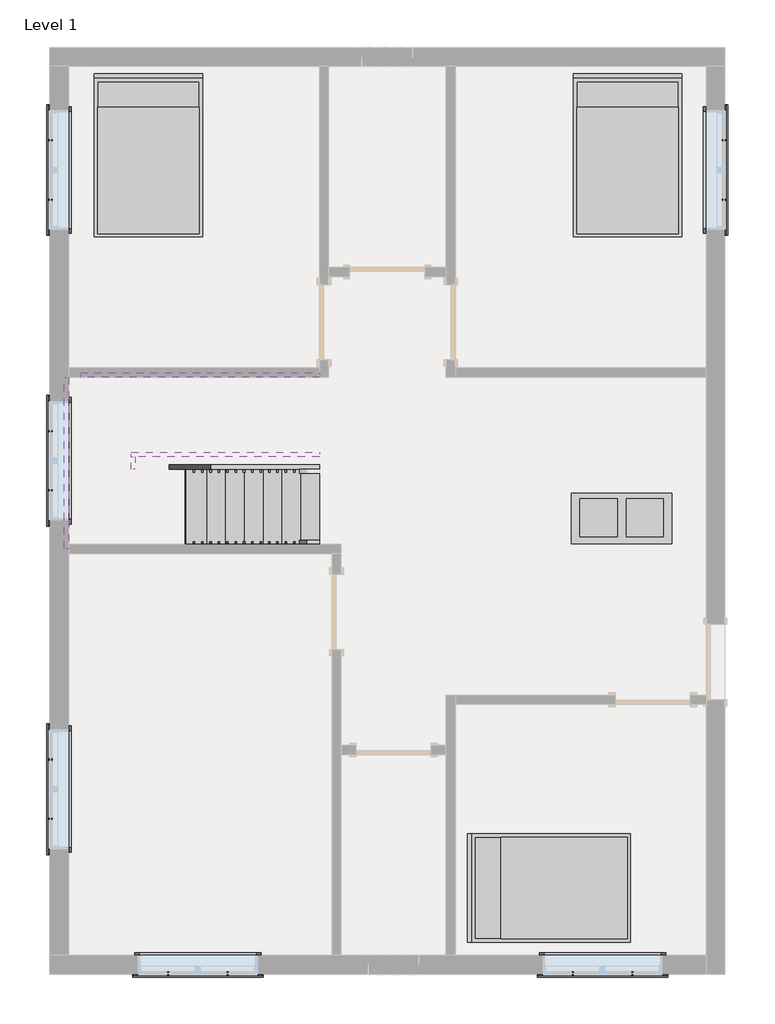
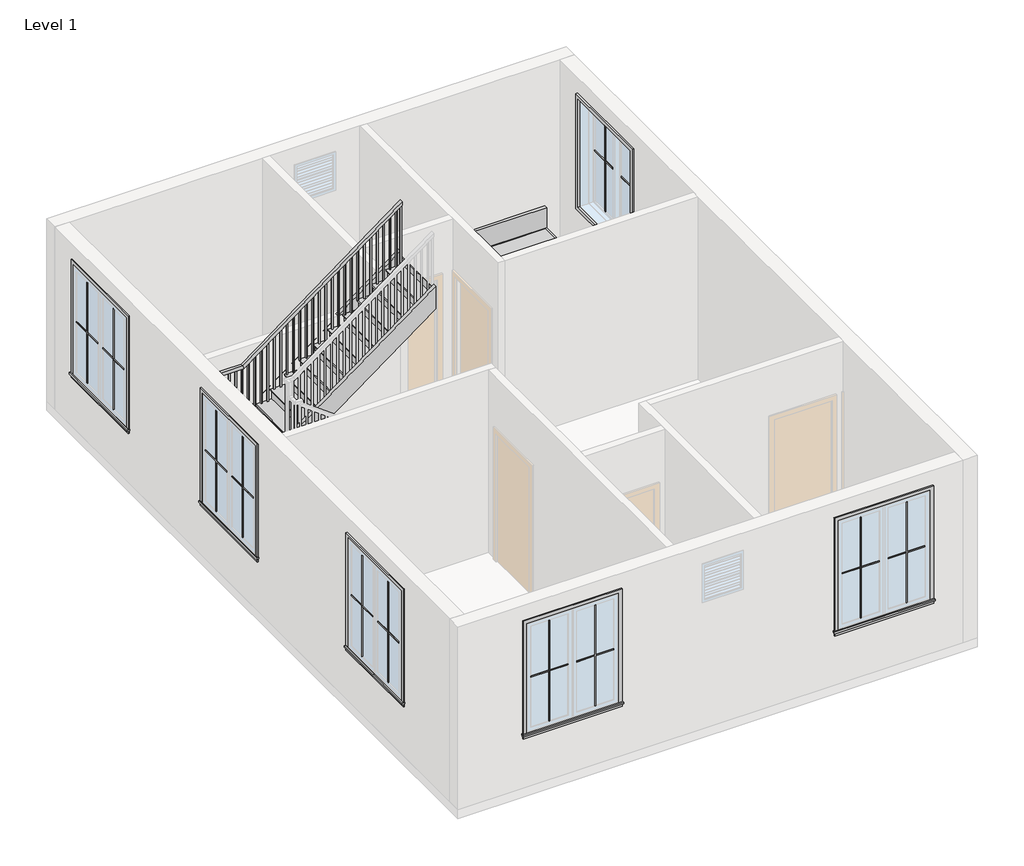
# One storey, part 2 of 2: 25 proxies, 6 members, 3 furniture elements, 1 railing, 1 stair flight.
"""IFC4 building model written with IfcOpenShell, lengths in millimetres."""

from ifc_helpers import new_model, si_unit, frame, origin, place, context, project, spatial, polyline, outline, extrude, faceted_brep, transform, mapped, element, save
from components import muntin_pattern_2x2_muntin_pattern_2x2_bff912c5, muntin_pattern_2x2_muntin_pattern_2x2_c2194282, trim_window_exterior_flat_with_sill_e04b3088, trim_window_interior_flat_picture_frame_2a7685fe, coffee_table_with_brass_mullions_11320_coffee_table_with_5962bef7, bed_17739_bed_17739_15c61121, stair_flight_66f938e6

model = new_model("IFC4")

# Units and contexts
model_context = context("Model", 3, world=origin())
ifc_project = project(units=[si_unit("LENGTHUNIT", "METRE", prefix="MILLI")], contexts=[model_context])

# Site, building, storey
site = spatial("IfcSite", under=ifc_project)
building = spatial("IfcBuilding", under=site)
storey = spatial("IfcBuildingStorey", under=building, Name="Level 1", Elevation=0.0)

# Proxies
placement = place(None, origin())
muntin_pattern_2x2_muntin_pattern_2x2_shape = muntin_pattern_2x2_muntin_pattern_2x2_bff912c5(model_context)
element("IfcBuildingElementProxy", 1, Name="Muntin Pattern_2x2 : Muntin Pattern_2x2", ObjectType="Muntin Pattern_2x2 : Muntin Pattern_2x2", at=placement, inside=storey, context=model_context, shape_type="MappedRepresentation", body=[
    mapped(muntin_pattern_2x2_muntin_pattern_2x2_shape, transform((-3196.8535855, -5792.3946383, 984.25), x_axis=(-1.0, 0.0, 0.0), y_axis=(0.0, -1.0, 0.0), z_axis=(0.0, 0.0, 1.0))),
])
element("IfcBuildingElementProxy", 2, Name="Muntin Pattern_2x2 : Muntin Pattern_2x2", ObjectType="Muntin Pattern_2x2 : Muntin Pattern_2x2", at=placement, inside=storey, context=model_context, shape_type="MappedRepresentation", body=[
    mapped(muntin_pattern_2x2_muntin_pattern_2x2_shape, transform((-5347.9160855, -3914.3821383, 984.25), x_axis=(0.0, 1.0, 0.0), y_axis=(-1.0, 0.0, 0.0), z_axis=(0.0, 0.0, 1.0))),
])
element("IfcBuildingElementProxy", 3, Name="Muntin Pattern_2x2 : Muntin Pattern_2x2", ObjectType="Muntin Pattern_2x2 : Muntin Pattern_2x2", at=placement, inside=storey, context=model_context, shape_type="MappedRepresentation", body=[
    mapped(muntin_pattern_2x2_muntin_pattern_2x2_shape, transform((1721.2214145, -5792.3946383, 984.25), x_axis=(-1.0, 0.0, 0.0), y_axis=(0.0, -1.0, 0.0), z_axis=(0.0, 0.0, 1.0))),
])
element("IfcBuildingElementProxy", 4, Name="Muntin Pattern_2x2 : Muntin Pattern_2x2", ObjectType="Muntin Pattern_2x2 : Muntin Pattern_2x2", at=placement, inside=storey, context=model_context, shape_type="MappedRepresentation", body=[
    mapped(muntin_pattern_2x2_muntin_pattern_2x2_shape, transform((2837.2339145, 4324.7428617, 984.25), x_axis=(0.0, -1.0, 0.0), y_axis=(1.0, 0.0, 0.0), z_axis=(0.0, 0.0, 1.0))),
])
element("IfcBuildingElementProxy", 5, Name="Muntin Pattern_2x2 : Muntin Pattern_2x2", ObjectType="Muntin Pattern_2x2 : Muntin Pattern_2x2", at=placement, inside=storey, context=model_context, shape_type="MappedRepresentation", body=[
    mapped(muntin_pattern_2x2_muntin_pattern_2x2_shape, transform((-5347.9160855, 3604.0178617, 984.25), x_axis=(0.0, 1.0, 0.0), y_axis=(-1.0, 0.0, 0.0), z_axis=(0.0, 0.0, 1.0))),
])
element("IfcBuildingElementProxy", 6, Name="Muntin Pattern_2x2 : Muntin Pattern_2x2", ObjectType="Muntin Pattern_2x2 : Muntin Pattern_2x2", at=placement, inside=storey, context=model_context, shape_type="MappedRepresentation", body=[
    mapped(muntin_pattern_2x2_muntin_pattern_2x2_shape, transform((-5347.9160855, 73.4178617, 984.25), x_axis=(0.0, 1.0, 0.0), y_axis=(-1.0, 0.0, 0.0), z_axis=(0.0, 0.0, 1.0))),
])
muntin_pattern_2x2_muntin_pattern_2x2_2_shape = muntin_pattern_2x2_muntin_pattern_2x2_c2194282(model_context)
element("IfcBuildingElementProxy", 7, Name="Muntin Pattern_2x2 : Muntin Pattern_2x2", ObjectType="Muntin Pattern_2x2 : Muntin Pattern_2x2", at=placement, inside=storey, context=model_context, shape_type="MappedRepresentation", body=[
    mapped(muntin_pattern_2x2_muntin_pattern_2x2_2_shape, transform((-3917.5785855, -5792.3946383, 984.25), x_axis=(1.0, 0.0, 0.0), y_axis=(0.0, 1.0, 0.0), z_axis=(0.0, 0.0, 1.0))),
])
element("IfcBuildingElementProxy", 8, Name="Muntin Pattern_2x2 : Muntin Pattern_2x2", ObjectType="Muntin Pattern_2x2 : Muntin Pattern_2x2", at=placement, inside=storey, context=model_context, shape_type="MappedRepresentation", body=[
    mapped(muntin_pattern_2x2_muntin_pattern_2x2_2_shape, transform((-5347.9160855, -3193.6571383, 984.25), x_axis=(0.0, -1.0, 0.0), y_axis=(1.0, 0.0, 0.0), z_axis=(0.0, 0.0, 1.0))),
])
element("IfcBuildingElementProxy", 9, Name="Muntin Pattern_2x2 : Muntin Pattern_2x2", ObjectType="Muntin Pattern_2x2 : Muntin Pattern_2x2", at=placement, inside=storey, context=model_context, shape_type="MappedRepresentation", body=[
    mapped(muntin_pattern_2x2_muntin_pattern_2x2_2_shape, transform((1000.4964145, -5792.3946383, 984.25), x_axis=(1.0, 0.0, 0.0), y_axis=(0.0, 1.0, 0.0), z_axis=(0.0, 0.0, 1.0))),
])
element("IfcBuildingElementProxy", 10, Name="Muntin Pattern_2x2 : Muntin Pattern_2x2", ObjectType="Muntin Pattern_2x2 : Muntin Pattern_2x2", at=placement, inside=storey, context=model_context, shape_type="MappedRepresentation", body=[
    mapped(muntin_pattern_2x2_muntin_pattern_2x2_2_shape, transform((2837.2339145, 3604.0178617, 984.25), x_axis=(0.0, 1.0, 0.0), y_axis=(-1.0, 0.0, 0.0), z_axis=(0.0, 0.0, 1.0))),
])
element("IfcBuildingElementProxy", 11, Name="Muntin Pattern_2x2 : Muntin Pattern_2x2", ObjectType="Muntin Pattern_2x2 : Muntin Pattern_2x2", at=placement, inside=storey, context=model_context, shape_type="MappedRepresentation", body=[
    mapped(muntin_pattern_2x2_muntin_pattern_2x2_2_shape, transform((-5347.9160855, 4324.7428617, 984.25), x_axis=(0.0, -1.0, 0.0), y_axis=(1.0, 0.0, 0.0), z_axis=(0.0, 0.0, 1.0))),
])
element("IfcBuildingElementProxy", 12, Name="Muntin Pattern_2x2 : Muntin Pattern_2x2", ObjectType="Muntin Pattern_2x2 : Muntin Pattern_2x2", at=placement, inside=storey, context=model_context, shape_type="MappedRepresentation", body=[
    mapped(muntin_pattern_2x2_muntin_pattern_2x2_2_shape, transform((-5347.9160855, 794.1428617, 984.25), x_axis=(0.0, -1.0, 0.0), y_axis=(1.0, 0.0, 0.0), z_axis=(0.0, 0.0, 1.0))),
])
trim_window_exterior_flat_with_sill_shape = trim_window_exterior_flat_with_sill_e04b3088(model_context)
element("IfcBuildingElementProxy", 13, Name="Trim-Window-Exterior-Flat : with Sill", ObjectType="Trim-Window-Exterior-Flat : with Sill", at=placement, inside=storey, context=model_context, shape_type="MappedRepresentation", body=[
    mapped(trim_window_exterior_flat_with_sill_shape, transform((-3557.2160855, -5801.9196383, 2743.2), x_axis=(1.0, 0.0, 0.0), y_axis=(0.0, 0.0, 1.0), z_axis=(0.0, -1.0, 0.0))),
])
element("IfcBuildingElementProxy", 14, Name="Trim-Window-Exterior-Flat : with Sill", ObjectType="Trim-Window-Exterior-Flat : with Sill", at=placement, inside=storey, context=model_context, shape_type="MappedRepresentation", body=[
    mapped(trim_window_exterior_flat_with_sill_shape, transform((-5357.4410855, -3554.0196383, 2743.2), x_axis=(0.0, -1.0, 0.0), y_axis=(0.0, 0.0, 1.0), z_axis=(-1.0, 0.0, 0.0))),
])
element("IfcBuildingElementProxy", 15, Name="Trim-Window-Exterior-Flat : with Sill", ObjectType="Trim-Window-Exterior-Flat : with Sill", at=placement, inside=storey, context=model_context, shape_type="MappedRepresentation", body=[
    mapped(trim_window_exterior_flat_with_sill_shape, transform((1360.8589145, -5801.9196383, 2743.2), x_axis=(1.0, 0.0, 0.0), y_axis=(0.0, 0.0, 1.0), z_axis=(0.0, -1.0, 0.0))),
])
element("IfcBuildingElementProxy", 16, Name="Trim-Window-Exterior-Flat : with Sill", ObjectType="Trim-Window-Exterior-Flat : with Sill", at=placement, inside=storey, context=model_context, shape_type="MappedRepresentation", body=[
    mapped(trim_window_exterior_flat_with_sill_shape, transform((2846.7589145, 3964.3803617, 2743.2), x_axis=(0.0, 1.0, 0.0), y_axis=(0.0, 0.0, 1.0), z_axis=(1.0, 0.0, 0.0))),
])
element("IfcBuildingElementProxy", 17, Name="Trim-Window-Exterior-Flat : with Sill", ObjectType="Trim-Window-Exterior-Flat : with Sill", at=placement, inside=storey, context=model_context, shape_type="MappedRepresentation", body=[
    mapped(trim_window_exterior_flat_with_sill_shape, transform((-5357.4410855, 3964.3803617, 2743.2), x_axis=(0.0, -1.0, 0.0), y_axis=(0.0, 0.0, 1.0), z_axis=(-1.0, 0.0, 0.0))),
])
element("IfcBuildingElementProxy", 18, Name="Trim-Window-Exterior-Flat : with Sill", ObjectType="Trim-Window-Exterior-Flat : with Sill", at=placement, inside=storey, context=model_context, shape_type="MappedRepresentation", body=[
    mapped(trim_window_exterior_flat_with_sill_shape, transform((-5357.4410855, 433.7803617, 2743.2), x_axis=(0.0, -1.0, 0.0), y_axis=(0.0, 0.0, 1.0), z_axis=(-1.0, 0.0, 0.0))),
])
trim_window_interior_flat_picture_frame_shape = trim_window_interior_flat_picture_frame_2a7685fe(model_context)
element("IfcBuildingElementProxy", 19, Name="Trim-Window-Interior-Flat : Picture Frame", ObjectType="Trim-Window-Interior-Flat : Picture Frame", at=placement, inside=storey, context=model_context, shape_type="MappedRepresentation", body=[
    mapped(trim_window_interior_flat_picture_frame_shape, transform((-3557.2160855, -5573.3196383, 2743.2), x_axis=(-1.0, 0.0, 0.0), y_axis=(0.0, 0.0, 1.0), z_axis=(0.0, 1.0, 0.0))),
])
element("IfcBuildingElementProxy", 20, Name="Trim-Window-Interior-Flat : Picture Frame", ObjectType="Trim-Window-Interior-Flat : Picture Frame", at=placement, inside=storey, context=model_context, shape_type="MappedRepresentation", body=[
    mapped(trim_window_interior_flat_picture_frame_shape, transform((-5128.8410855, -3554.0196383, 2743.2), x_axis=(0.0, 1.0, 0.0), y_axis=(0.0, 0.0, 1.0), z_axis=(1.0, 0.0, 0.0))),
])
element("IfcBuildingElementProxy", 21, Name="Trim-Window-Interior-Flat : Picture Frame", ObjectType="Trim-Window-Interior-Flat : Picture Frame", at=placement, inside=storey, context=model_context, shape_type="MappedRepresentation", body=[
    mapped(trim_window_interior_flat_picture_frame_shape, transform((1360.8589145, -5573.3196383, 2743.2), x_axis=(-1.0, 0.0, 0.0), y_axis=(0.0, 0.0, 1.0), z_axis=(0.0, 1.0, 0.0))),
])
element("IfcBuildingElementProxy", 22, Name="Trim-Window-Interior-Flat : Picture Frame", ObjectType="Trim-Window-Interior-Flat : Picture Frame", at=placement, inside=storey, context=model_context, shape_type="MappedRepresentation", body=[
    mapped(trim_window_interior_flat_picture_frame_shape, transform((2618.1589145, 3964.3803617, 2743.2), x_axis=(0.0, -1.0, 0.0), y_axis=(0.0, 0.0, 1.0), z_axis=(-1.0, 0.0, 0.0))),
])
element("IfcBuildingElementProxy", 23, Name="Trim-Window-Interior-Flat : Picture Frame", ObjectType="Trim-Window-Interior-Flat : Picture Frame", at=placement, inside=storey, context=model_context, shape_type="MappedRepresentation", body=[
    mapped(trim_window_interior_flat_picture_frame_shape, transform((-5128.8410855, 3964.3803617, 2743.2), x_axis=(0.0, 1.0, 0.0), y_axis=(0.0, 0.0, 1.0), z_axis=(1.0, 0.0, 0.0))),
])
element("IfcBuildingElementProxy", 24, Name="Trim-Window-Interior-Flat : Picture Frame", ObjectType="Trim-Window-Interior-Flat : Picture Frame", at=placement, inside=storey, context=model_context, shape_type="MappedRepresentation", body=[
    mapped(trim_window_interior_flat_picture_frame_shape, transform((-5128.8410855, 433.7803617, 2743.2), x_axis=(0.0, 1.0, 0.0), y_axis=(0.0, 0.0, 1.0), z_axis=(1.0, 0.0, 0.0))),
])
coffee_table_with_brass_mullions_11320_coffee_table_with_shape = coffee_table_with_brass_mullions_11320_coffee_table_with_5962bef7(model_context)
element("IfcBuildingElementProxy", 25, Name="coffee_table_with_brass_mullions_11320 : coffee_table_with_brass_mullions_11320", ObjectType="coffee_table_with_brass_mullions_11320 : coffee_table_with_brass_mullions_11320", at=placement, inside=storey, context=model_context, shape_type="MappedRepresentation", body=[
    mapped(coffee_table_with_brass_mullions_11320_coffee_table_with_shape, transform((2229.2258874, -696.5196383, 0.0), x_axis=(1.0, 0.0, 0.0), y_axis=(0.0, 1.0, 0.0), z_axis=(0.0, 0.0, 1.0))),
])

# Furniture
bed_17739_bed_17739_shape = bed_17739_bed_17739_15c61121(model_context)
element("IfcFurniture", 26, ObjectType="Bed_17739 : Bed_17739", at=placement, inside=storey, context=model_context, shape_type="MappedRepresentation", body=[
    mapped(bed_17739_bed_17739_shape, transform((1665.6589145, 4116.7803617, 0.0), x_axis=(1.0, 0.0, 0.0), y_axis=(0.0, 1.0, 0.0), z_axis=(0.0, 0.0, 1.0))),
])
element("IfcFurniture", 27, ObjectType="Bed_17739 : Bed_17739", at=placement, inside=storey, context=model_context, shape_type="MappedRepresentation", body=[
    mapped(bed_17739_bed_17739_shape, transform((-4157.2910855, 4116.7803617, 0.0), x_axis=(1.0, 0.0, 0.0), y_axis=(0.0, 1.0, 0.0), z_axis=(0.0, 0.0, 1.0))),
])
element("IfcFurniture", 28, ObjectType="Bed_17739 : Bed_17739", at=placement, inside=storey, context=model_context, shape_type="MappedRepresentation", body=[
    mapped(bed_17739_bed_17739_shape, transform((732.2089145, -4754.5725945, 0.0), x_axis=(0.0, 1.0, 0.0), y_axis=(-1.0, 0.0, 0.0), z_axis=(0.0, 0.0, 1.0))),
])

# Members
element("IfcMember", 29, ObjectType="Stringer - 2\" Width", at=placement, inside=storey, context=model_context, shape_type="SweptSolid", body=[
    extrude(outline(polyline([(0.0, -2080.8410855), (225.9712455, -2080.8410855), (1938.8666667, -4393.249904), (1938.8666667, -4905.3229753), (0.0, -2287.8529753), (0.0, -2080.8410855)])), frame((0.0, -633.0196383, 0.0), z_axis=(0.0, 1.0, 0.0), x_axis=(0.0, 0.0, 1.0)), (0.0, 0.0, 1.0), 50.8),
])
element("IfcMember", 30, ObjectType="Stringer - 2\" Width", at=placement, inside=storey, context=model_context, shape_type="SweptSolid", body=[
    extrude(outline(polyline([(-5128.8410855, -633.0196383), (-5179.6410855, -633.0196383), (-5179.6410855, 1449.7803617), (-5128.8410855, 1449.7803617), (-5128.8410855, -633.0196383)])), frame((0.0, 0.0, 1634.0666667), z_axis=(0.0, 0.0, 1.0), x_axis=(1.0, 0.0, 0.0)), (0.0, 0.0, 1.0), 304.8),
])
element("IfcMember", 31, ObjectType="Stringer - 2\" Width", at=placement, inside=storey, context=model_context, shape_type="SweptSolid", body=[
    extrude(outline(polyline([(1634.0666667, -4468.4391956), (3402.6578594, -2080.8410855), (3781.9712455, -2080.8410855), (1634.0666667, -4980.512267), (1634.0666667, -4468.4391956)])), frame((0.0, 1449.7803617, 0.0), z_axis=(0.0, 1.0, 0.0), x_axis=(0.0, 0.0, 1.0)), (0.0, 0.0, 1.0), 50.8),
])
element("IfcMember", 32, ObjectType="Stringer - 2\" Width", at=placement, inside=storey, context=model_context, shape_type="SweptSolid", body=[
    extrude(outline(polyline([(0.0, -2080.8410855), (225.9712455, -2080.8410855), (1881.6749492, -4316.0410855), (1502.3615631, -4316.0410855), (0.0, -2287.8529753), (0.0, -2080.8410855)])), frame((0.0, 332.1803617, 0.0), z_axis=(0.0, 1.0, 0.0), x_axis=(0.0, 0.0, 1.0)), (0.0, 0.0, 1.0), 50.8),
])
element("IfcMember", 33, ObjectType="Stringer - 2\" Width", at=placement, inside=storey, context=model_context, shape_type="SweptSolid", body=[
    extrude(outline(polyline([(-4316.0410855, 332.1803617), (-4366.8410855, 332.1803617), (-4366.8410855, 484.5803617), (-4316.0410855, 484.5803617), (-4316.0410855, 332.1803617)])), frame((0.0, 0.0, 1634.0666667), z_axis=(0.0, 0.0, 1.0), x_axis=(1.0, 0.0, 0.0)), (0.0, 0.0, 1.0), 304.8),
])
element("IfcMember", 34, ObjectType="Stringer - 2\" Width", at=placement, inside=storey, context=model_context, shape_type="SweptSolid", body=[
    extrude(outline(polyline([(2088.6379122, -4366.8410855), (1709.324526, -4366.8410855), (3402.6578594, -2080.8410855), (3781.9712455, -2080.8410855), (2088.6379122, -4366.8410855)])), frame((0.0, 484.5803617, 0.0), z_axis=(0.0, 1.0, 0.0), x_axis=(0.0, 0.0, 1.0)), (0.0, 0.0, 1.0), 50.8),
])

# Railing
element("IfcRailing", 35, ObjectType="Handrail - Rectangular", at=placement, inside=storey, context=model_context, shape_type="SolidModel", body=[
    faceted_brep([(-2080.8410855, -582.2196383, 1083.7333333), (-2080.8410855, -582.2196383, 1020.5144356), (-2080.8410855, -531.4196383, 1020.5144356), (-2080.8410855, -531.4196383, 1083.7333333), (-4366.8410855, -582.2196383, 2777.0666667), (-4383.6065974, -582.2196383, 2726.2666667), (-4383.6065974, -531.4196383, 2726.2666667), (-4366.8410855, -531.4196383, 2777.0666667), (-5128.8410855, -582.2196383, 2777.0666667), (-5128.8410855, -582.2196383, 2726.2666667), (-5078.0410855, -531.4196383, 2726.2666667), (-5078.0410855, -531.4196383, 2777.0666667), (-5128.8410855, 1449.7803617, 2777.0666667), (-5128.8410855, 1449.7803617, 2726.2666667), (-5078.0410855, 1398.9803617, 2726.2666667), (-5078.0410855, 1398.9803617, 2777.0666667), (-4595.4410855, 1449.7803617, 2777.0666667), (-4578.6755736, 1449.7803617, 2726.2666667), (-4578.6755736, 1398.9803617, 2726.2666667), (-4595.4410855, 1398.9803617, 2777.0666667), (-2080.8410855, 1449.7803617, 4639.7333333), (-2080.8410855, 1398.9803617, 4639.7333333), (-2080.8410855, 1398.9803617, 4576.5144356), (-2080.8410855, 1449.7803617, 4576.5144356)], [[[0, 1, 2, 3]], [[1, 0, 4, 5]], [[2, 1, 5, 6]], [[3, 2, 6, 7]], [[0, 3, 7, 4]], [[5, 4, 8, 9]], [[6, 5, 9, 10]], [[7, 6, 10, 11]], [[4, 7, 11, 8]], [[9, 8, 12, 13]], [[10, 9, 13, 14]], [[11, 10, 14, 15]], [[8, 11, 15, 12]], [[13, 12, 16, 17]], [[14, 13, 17, 18]], [[15, 14, 18, 19]], [[12, 15, 19, 16]], [[20, 21, 22, 23]], [[17, 16, 20, 23]], [[18, 17, 23, 22]], [[19, 18, 22, 21]], [[16, 19, 21, 20]]]),
    extrude(outline(polyline([(4513.0144356, -2166.5660855), (3556.0, -2166.5660855), (3556.0, -2147.5160855), (4527.1255467, -2147.5160855), (4513.0144356, -2166.5660855)])), frame((0.0, 1414.8553617, 0.0), z_axis=(0.0, 1.0, 0.0), x_axis=(0.0, 0.0, 1.0)), (0.0, 0.0, 1.0), 19.05),
    extrude(outline(polyline([(4437.7551764, -2268.1660855), (3556.0, -2268.1660855), (3556.0, -2249.1160855), (4451.8662875, -2249.1160855), (4437.7551764, -2268.1660855)])), frame((0.0, 1414.8553617, 0.0), z_axis=(0.0, 1.0, 0.0), x_axis=(0.0, 0.0, 1.0)), (0.0, 0.0, 1.0), 19.05),
    extrude(outline(polyline([(4362.4959171, -2369.7660855), (3386.6666667, -2369.7660855), (3386.6666667, -2350.7160855), (4376.6070282, -2350.7160855), (4362.4959171, -2369.7660855)])), frame((0.0, 1414.8553617, 0.0), z_axis=(0.0, 1.0, 0.0), x_axis=(0.0, 0.0, 1.0)), (0.0, 0.0, 1.0), 19.05),
    extrude(outline(polyline([(4287.2366579, -2471.3660855), (3386.6666667, -2471.3660855), (3386.6666667, -2452.3160855), (4301.347769, -2452.3160855), (4287.2366579, -2471.3660855)])), frame((0.0, 1414.8553617, 0.0), z_axis=(0.0, 1.0, 0.0), x_axis=(0.0, 0.0, 1.0)), (0.0, 0.0, 1.0), 19.05),
    extrude(outline(polyline([(4211.9773986, -2572.9660855), (3217.3333333, -2572.9660855), (3217.3333333, -2553.9160855), (4226.0885097, -2553.9160855), (4211.9773986, -2572.9660855)])), frame((0.0, 1414.8553617, 0.0), z_axis=(0.0, 1.0, 0.0), x_axis=(0.0, 0.0, 1.0)), (0.0, 0.0, 1.0), 19.05),
    extrude(outline(polyline([(4136.7181393, -2674.5660855), (3217.3333333, -2674.5660855), (3217.3333333, -2655.5160855), (4150.8292505, -2655.5160855), (4136.7181393, -2674.5660855)])), frame((0.0, 1414.8553617, 0.0), z_axis=(0.0, 1.0, 0.0), x_axis=(0.0, 0.0, 1.0)), (0.0, 0.0, 1.0), 19.05),
    extrude(outline(polyline([(4061.4588801, -2776.1660855), (3217.3333333, -2776.1660855), (3217.3333333, -2757.1160855), (4075.5699912, -2757.1160855), (4061.4588801, -2776.1660855)])), frame((0.0, 1414.8553617, 0.0), z_axis=(0.0, 1.0, 0.0), x_axis=(0.0, 0.0, 1.0)), (0.0, 0.0, 1.0), 19.05),
    extrude(outline(polyline([(3986.1996208, -2877.7660855), (3048.0, -2877.7660855), (3048.0, -2858.7160855), (4000.3107319, -2858.7160855), (3986.1996208, -2877.7660855)])), frame((0.0, 1414.8553617, 0.0), z_axis=(0.0, 1.0, 0.0), x_axis=(0.0, 0.0, 1.0)), (0.0, 0.0, 1.0), 19.05),
    extrude(outline(polyline([(3910.9403616, -2979.3660855), (3048.0, -2979.3660855), (3048.0, -2960.3160855), (3925.0514727, -2960.3160855), (3910.9403616, -2979.3660855)])), frame((0.0, 1414.8553617, 0.0), z_axis=(0.0, 1.0, 0.0), x_axis=(0.0, 0.0, 1.0)), (0.0, 0.0, 1.0), 19.05),
    extrude(outline(polyline([(3835.6811023, -3080.9660855), (2878.6666667, -3080.9660855), (2878.6666667, -3061.9160855), (3849.7922134, -3061.9160855), (3835.6811023, -3080.9660855)])), frame((0.0, 1414.8553617, 0.0), z_axis=(0.0, 1.0, 0.0), x_axis=(0.0, 0.0, 1.0)), (0.0, 0.0, 1.0), 19.05),
    extrude(outline(polyline([(3760.421843, -3182.5660855), (2878.6666667, -3182.5660855), (2878.6666667, -3163.5160855), (3774.5329542, -3163.5160855), (3760.421843, -3182.5660855)])), frame((0.0, 1414.8553617, 0.0), z_axis=(0.0, 1.0, 0.0), x_axis=(0.0, 0.0, 1.0)), (0.0, 0.0, 1.0), 19.05),
    extrude(outline(polyline([(3685.1625838, -3284.1660855), (2709.3333333, -3284.1660855), (2709.3333333, -3265.1160855), (3699.2736949, -3265.1160855), (3685.1625838, -3284.1660855)])), frame((0.0, 1414.8553617, 0.0), z_axis=(0.0, 1.0, 0.0), x_axis=(0.0, 0.0, 1.0)), (0.0, 0.0, 1.0), 19.05),
    extrude(outline(polyline([(3609.9033245, -3385.7660855), (2709.3333333, -3385.7660855), (2709.3333333, -3366.7160855), (3624.0144356, -3366.7160855), (3609.9033245, -3385.7660855)])), frame((0.0, 1414.8553617, 0.0), z_axis=(0.0, 1.0, 0.0), x_axis=(0.0, 0.0, 1.0)), (0.0, 0.0, 1.0), 19.05),
    extrude(outline(polyline([(3534.6440653, -3487.3660855), (2540.0, -3487.3660855), (2540.0, -3468.3160855), (3548.7551764, -3468.3160855), (3534.6440653, -3487.3660855)])), frame((0.0, 1414.8553617, 0.0), z_axis=(0.0, 1.0, 0.0), x_axis=(0.0, 0.0, 1.0)), (0.0, 0.0, 1.0), 19.05),
    extrude(outline(polyline([(3459.384806, -3588.9660855), (2540.0, -3588.9660855), (2540.0, -3569.9160855), (3473.4959171, -3569.9160855), (3459.384806, -3588.9660855)])), frame((0.0, 1414.8553617, 0.0), z_axis=(0.0, 1.0, 0.0), x_axis=(0.0, 0.0, 1.0)), (0.0, 0.0, 1.0), 19.05),
    extrude(outline(polyline([(3384.1255467, -3690.5660855), (2540.0, -3690.5660855), (2540.0, -3671.5160855), (3398.2366579, -3671.5160855), (3384.1255467, -3690.5660855)])), frame((0.0, 1414.8553617, 0.0), z_axis=(0.0, 1.0, 0.0), x_axis=(0.0, 0.0, 1.0)), (0.0, 0.0, 1.0), 19.05),
    extrude(outline(polyline([(3308.8662875, -3792.1660855), (2370.6666667, -3792.1660855), (2370.6666667, -3773.1160855), (3322.9773986, -3773.1160855), (3308.8662875, -3792.1660855)])), frame((0.0, 1414.8553617, 0.0), z_axis=(0.0, 1.0, 0.0), x_axis=(0.0, 0.0, 1.0)), (0.0, 0.0, 1.0), 19.05),
    extrude(outline(polyline([(3233.6070282, -3893.7660855), (2370.6666667, -3893.7660855), (2370.6666667, -3874.7160855), (3247.7181393, -3874.7160855), (3233.6070282, -3893.7660855)])), frame((0.0, 1414.8553617, 0.0), z_axis=(0.0, 1.0, 0.0), x_axis=(0.0, 0.0, 1.0)), (0.0, 0.0, 1.0), 19.05),
    extrude(outline(polyline([(3158.347769, -3995.3660855), (2201.3333333, -3995.3660855), (2201.3333333, -3976.3160855), (3172.4588801, -3976.3160855), (3158.347769, -3995.3660855)])), frame((0.0, 1414.8553617, 0.0), z_axis=(0.0, 1.0, 0.0), x_axis=(0.0, 0.0, 1.0)), (0.0, 0.0, 1.0), 19.05),
    extrude(outline(polyline([(3083.0885097, -4096.9660855), (2201.3333333, -4096.9660855), (2201.3333333, -4077.9160855), (3097.1996208, -4077.9160855), (3083.0885097, -4096.9660855)])), frame((0.0, 1414.8553617, 0.0), z_axis=(0.0, 1.0, 0.0), x_axis=(0.0, 0.0, 1.0)), (0.0, 0.0, 1.0), 19.05),
    extrude(outline(polyline([(3007.8292505, -4198.5660855), (2032.0, -4198.5660855), (2032.0, -4179.5160855), (3021.9403616, -4179.5160855), (3007.8292505, -4198.5660855)])), frame((0.0, 1414.8553617, 0.0), z_axis=(0.0, 1.0, 0.0), x_axis=(0.0, 0.0, 1.0)), (0.0, 0.0, 1.0), 19.05),
    extrude(outline(polyline([(2932.5699912, -4300.1660855), (2032.0, -4300.1660855), (2032.0, -4281.1160855), (2946.6811023, -4281.1160855), (2932.5699912, -4300.1660855)])), frame((0.0, 1414.8553617, 0.0), z_axis=(0.0, 1.0, 0.0), x_axis=(0.0, 0.0, 1.0)), (0.0, 0.0, 1.0), 19.05),
    extrude(outline(polyline([(2857.3107319, -4401.7660855), (1862.6666667, -4401.7660855), (1862.6666667, -4382.7160855), (2871.421843, -4382.7160855), (2857.3107319, -4401.7660855)])), frame((0.0, 1414.8553617, 0.0), z_axis=(0.0, 1.0, 0.0), x_axis=(0.0, 0.0, 1.0)), (0.0, 0.0, 1.0), 19.05),
    extrude(outline(polyline([(2782.0514727, -4503.3660855), (1862.6666667, -4503.3660855), (1862.6666667, -4484.3160855), (2796.1625838, -4484.3160855), (2782.0514727, -4503.3660855)])), frame((0.0, 1414.8553617, 0.0), z_axis=(0.0, 1.0, 0.0), x_axis=(0.0, 0.0, 1.0)), (0.0, 0.0, 1.0), 19.05),
    extrude(outline(polyline([(-4604.9660855, 1433.9053617), (-4585.9160855, 1433.9053617), (-4585.9160855, 1414.8553617), (-4604.9660855, 1414.8553617), (-4604.9660855, 1433.9053617)])), frame((0.0, 0.0, 1862.6666667), z_axis=(0.0, 0.0, 1.0), x_axis=(1.0, 0.0, 0.0)), (0.0, 0.0, 1.0), 863.6),
    extrude(outline(polyline([(-4706.5660855, 1433.9053617), (-4687.5160855, 1433.9053617), (-4687.5160855, 1414.8553617), (-4706.5660855, 1414.8553617), (-4706.5660855, 1433.9053617)])), frame((0.0, 0.0, 1862.6666667), z_axis=(0.0, 0.0, 1.0), x_axis=(1.0, 0.0, 0.0)), (0.0, 0.0, 1.0), 863.6),
    extrude(outline(polyline([(-4808.1660855, 1433.9053617), (-4789.1160855, 1433.9053617), (-4789.1160855, 1414.8553617), (-4808.1660855, 1414.8553617), (-4808.1660855, 1433.9053617)])), frame((0.0, 0.0, 1862.6666667), z_axis=(0.0, 0.0, 1.0), x_axis=(1.0, 0.0, 0.0)), (0.0, 0.0, 1.0), 863.6),
    extrude(outline(polyline([(-4909.7660855, 1433.9053617), (-4890.7160855, 1433.9053617), (-4890.7160855, 1414.8553617), (-4909.7660855, 1414.8553617), (-4909.7660855, 1433.9053617)])), frame((0.0, 0.0, 1862.6666667), z_axis=(0.0, 0.0, 1.0), x_axis=(1.0, 0.0, 0.0)), (0.0, 0.0, 1.0), 863.6),
    extrude(outline(polyline([(-5011.3660855, 1433.9053617), (-4992.3160855, 1433.9053617), (-4992.3160855, 1414.8553617), (-5011.3660855, 1414.8553617), (-5011.3660855, 1433.9053617)])), frame((0.0, 0.0, 1862.6666667), z_axis=(0.0, 0.0, 1.0), x_axis=(1.0, 0.0, 0.0)), (0.0, 0.0, 1.0), 863.6),
    extrude(outline(polyline([(-5112.9660855, 1364.0553617), (-5112.9660855, 1383.1053617), (-5093.9160855, 1383.1053617), (-5093.9160855, 1364.0553617), (-5112.9660855, 1364.0553617)])), frame((0.0, 0.0, 1862.6666667), z_axis=(0.0, 0.0, 1.0), x_axis=(1.0, 0.0, 0.0)), (0.0, 0.0, 1.0), 863.6),
    extrude(outline(polyline([(-5112.9660855, 1262.4553617), (-5112.9660855, 1281.5053617), (-5093.9160855, 1281.5053617), (-5093.9160855, 1262.4553617), (-5112.9660855, 1262.4553617)])), frame((0.0, 0.0, 1862.6666667), z_axis=(0.0, 0.0, 1.0), x_axis=(1.0, 0.0, 0.0)), (0.0, 0.0, 1.0), 863.6),
    extrude(outline(polyline([(-5112.9660855, 1160.8553617), (-5112.9660855, 1179.9053617), (-5093.9160855, 1179.9053617), (-5093.9160855, 1160.8553617), (-5112.9660855, 1160.8553617)])), frame((0.0, 0.0, 1862.6666667), z_axis=(0.0, 0.0, 1.0), x_axis=(1.0, 0.0, 0.0)), (0.0, 0.0, 1.0), 863.6),
    extrude(outline(polyline([(-5112.9660855, 1059.2553617), (-5112.9660855, 1078.3053617), (-5093.9160855, 1078.3053617), (-5093.9160855, 1059.2553617), (-5112.9660855, 1059.2553617)])), frame((0.0, 0.0, 1862.6666667), z_axis=(0.0, 0.0, 1.0), x_axis=(1.0, 0.0, 0.0)), (0.0, 0.0, 1.0), 863.6),
    extrude(outline(polyline([(-5112.9660855, 957.6553617), (-5112.9660855, 976.7053617), (-5093.9160855, 976.7053617), (-5093.9160855, 957.6553617), (-5112.9660855, 957.6553617)])), frame((0.0, 0.0, 1862.6666667), z_axis=(0.0, 0.0, 1.0), x_axis=(1.0, 0.0, 0.0)), (0.0, 0.0, 1.0), 863.6),
    extrude(outline(polyline([(-5112.9660855, 856.0553617), (-5112.9660855, 875.1053617), (-5093.9160855, 875.1053617), (-5093.9160855, 856.0553617), (-5112.9660855, 856.0553617)])), frame((0.0, 0.0, 1862.6666667), z_axis=(0.0, 0.0, 1.0), x_axis=(1.0, 0.0, 0.0)), (0.0, 0.0, 1.0), 863.6),
    extrude(outline(polyline([(-5112.9660855, 754.4553617), (-5112.9660855, 773.5053617), (-5093.9160855, 773.5053617), (-5093.9160855, 754.4553617), (-5112.9660855, 754.4553617)])), frame((0.0, 0.0, 1862.6666667), z_axis=(0.0, 0.0, 1.0), x_axis=(1.0, 0.0, 0.0)), (0.0, 0.0, 1.0), 863.6),
    extrude(outline(polyline([(-5112.9660855, 652.8553617), (-5112.9660855, 671.9053617), (-5093.9160855, 671.9053617), (-5093.9160855, 652.8553617), (-5112.9660855, 652.8553617)])), frame((0.0, 0.0, 1862.6666667), z_axis=(0.0, 0.0, 1.0), x_axis=(1.0, 0.0, 0.0)), (0.0, 0.0, 1.0), 863.6),
    extrude(outline(polyline([(-5112.9660855, 551.2553617), (-5112.9660855, 570.3053617), (-5093.9160855, 570.3053617), (-5093.9160855, 551.2553617), (-5112.9660855, 551.2553617)])), frame((0.0, 0.0, 1862.6666667), z_axis=(0.0, 0.0, 1.0), x_axis=(1.0, 0.0, 0.0)), (0.0, 0.0, 1.0), 863.6),
    extrude(outline(polyline([(-5112.9660855, 449.6553617), (-5112.9660855, 468.7053617), (-5093.9160855, 468.7053617), (-5093.9160855, 449.6553617), (-5112.9660855, 449.6553617)])), frame((0.0, 0.0, 1862.6666667), z_axis=(0.0, 0.0, 1.0), x_axis=(1.0, 0.0, 0.0)), (0.0, 0.0, 1.0), 863.6),
    extrude(outline(polyline([(-5112.9660855, 348.0553617), (-5112.9660855, 367.1053617), (-5093.9160855, 367.1053617), (-5093.9160855, 348.0553617), (-5112.9660855, 348.0553617)])), frame((0.0, 0.0, 1862.6666667), z_axis=(0.0, 0.0, 1.0), x_axis=(1.0, 0.0, 0.0)), (0.0, 0.0, 1.0), 863.6),
    extrude(outline(polyline([(-5112.9660855, 246.4553617), (-5112.9660855, 265.5053617), (-5093.9160855, 265.5053617), (-5093.9160855, 246.4553617), (-5112.9660855, 246.4553617)])), frame((0.0, 0.0, 1862.6666667), z_axis=(0.0, 0.0, 1.0), x_axis=(1.0, 0.0, 0.0)), (0.0, 0.0, 1.0), 863.6),
    extrude(outline(polyline([(-5112.9660855, 144.8553617), (-5112.9660855, 163.9053617), (-5093.9160855, 163.9053617), (-5093.9160855, 144.8553617), (-5112.9660855, 144.8553617)])), frame((0.0, 0.0, 1862.6666667), z_axis=(0.0, 0.0, 1.0), x_axis=(1.0, 0.0, 0.0)), (0.0, 0.0, 1.0), 863.6),
    extrude(outline(polyline([(-5112.9660855, 43.2553617), (-5112.9660855, 62.3053617), (-5093.9160855, 62.3053617), (-5093.9160855, 43.2553617), (-5112.9660855, 43.2553617)])), frame((0.0, 0.0, 1862.6666667), z_axis=(0.0, 0.0, 1.0), x_axis=(1.0, 0.0, 0.0)), (0.0, 0.0, 1.0), 863.6),
    extrude(outline(polyline([(-5112.9660855, -58.3446383), (-5112.9660855, -39.2946383), (-5093.9160855, -39.2946383), (-5093.9160855, -58.3446383), (-5112.9660855, -58.3446383)])), frame((0.0, 0.0, 1862.6666667), z_axis=(0.0, 0.0, 1.0), x_axis=(1.0, 0.0, 0.0)), (0.0, 0.0, 1.0), 863.6),
    extrude(outline(polyline([(-5112.9660855, -159.9446383), (-5112.9660855, -140.8946383), (-5093.9160855, -140.8946383), (-5093.9160855, -159.9446383), (-5112.9660855, -159.9446383)])), frame((0.0, 0.0, 1862.6666667), z_axis=(0.0, 0.0, 1.0), x_axis=(1.0, 0.0, 0.0)), (0.0, 0.0, 1.0), 863.6),
    extrude(outline(polyline([(-5112.9660855, -261.5446383), (-5112.9660855, -242.4946383), (-5093.9160855, -242.4946383), (-5093.9160855, -261.5446383), (-5112.9660855, -261.5446383)])), frame((0.0, 0.0, 1862.6666667), z_axis=(0.0, 0.0, 1.0), x_axis=(1.0, 0.0, 0.0)), (0.0, 0.0, 1.0), 863.6),
    extrude(outline(polyline([(-5112.9660855, -363.1446383), (-5112.9660855, -344.0946383), (-5093.9160855, -344.0946383), (-5093.9160855, -363.1446383), (-5112.9660855, -363.1446383)])), frame((0.0, 0.0, 1862.6666667), z_axis=(0.0, 0.0, 1.0), x_axis=(1.0, 0.0, 0.0)), (0.0, 0.0, 1.0), 863.6),
    extrude(outline(polyline([(-5112.9660855, -464.7446383), (-5112.9660855, -445.6946383), (-5093.9160855, -445.6946383), (-5093.9160855, -464.7446383), (-5112.9660855, -464.7446383)])), frame((0.0, 0.0, 1862.6666667), z_axis=(0.0, 0.0, 1.0), x_axis=(1.0, 0.0, 0.0)), (0.0, 0.0, 1.0), 863.6),
    extrude(outline(polyline([(-5017.7160855, -566.3446383), (-5036.7660855, -566.3446383), (-5036.7660855, -547.2946383), (-5017.7160855, -547.2946383), (-5017.7160855, -566.3446383)])), frame((0.0, 0.0, 1862.6666667), z_axis=(0.0, 0.0, 1.0), x_axis=(1.0, 0.0, 0.0)), (0.0, 0.0, 1.0), 863.6),
    extrude(outline(polyline([(-4916.1160855, -566.3446383), (-4935.1660855, -566.3446383), (-4935.1660855, -547.2946383), (-4916.1160855, -547.2946383), (-4916.1160855, -566.3446383)])), frame((0.0, 0.0, 1862.6666667), z_axis=(0.0, 0.0, 1.0), x_axis=(1.0, 0.0, 0.0)), (0.0, 0.0, 1.0), 863.6),
    extrude(outline(polyline([(-4814.5160855, -566.3446383), (-4833.5660855, -566.3446383), (-4833.5660855, -547.2946383), (-4814.5160855, -547.2946383), (-4814.5160855, -566.3446383)])), frame((0.0, 0.0, 1862.6666667), z_axis=(0.0, 0.0, 1.0), x_axis=(1.0, 0.0, 0.0)), (0.0, 0.0, 1.0), 863.6),
    extrude(outline(polyline([(-4712.9160855, -566.3446383), (-4731.9660855, -566.3446383), (-4731.9660855, -547.2946383), (-4712.9160855, -547.2946383), (-4712.9160855, -566.3446383)])), frame((0.0, 0.0, 1862.6666667), z_axis=(0.0, 0.0, 1.0), x_axis=(1.0, 0.0, 0.0)), (0.0, 0.0, 1.0), 863.6),
    extrude(outline(polyline([(-4611.3160855, -566.3446383), (-4630.3660855, -566.3446383), (-4630.3660855, -547.2946383), (-4611.3160855, -547.2946383), (-4611.3160855, -566.3446383)])), frame((0.0, 0.0, 1862.6666667), z_axis=(0.0, 0.0, 1.0), x_axis=(1.0, 0.0, 0.0)), (0.0, 0.0, 1.0), 863.6),
    extrude(outline(polyline([(-4509.7160855, -566.3446383), (-4528.7660855, -566.3446383), (-4528.7660855, -547.2946383), (-4509.7160855, -547.2946383), (-4509.7160855, -566.3446383)])), frame((0.0, 0.0, 1862.6666667), z_axis=(0.0, 0.0, 1.0), x_axis=(1.0, 0.0, 0.0)), (0.0, 0.0, 1.0), 863.6),
    extrude(outline(polyline([(-4408.1160855, -566.3446383), (-4427.1660855, -566.3446383), (-4427.1660855, -547.2946383), (-4408.1160855, -547.2946383), (-4408.1160855, -566.3446383)])), frame((0.0, 0.0, 1862.6666667), z_axis=(0.0, 0.0, 1.0), x_axis=(1.0, 0.0, 0.0)), (0.0, 0.0, 1.0), 863.6),
    extrude(outline(polyline([(2683.2736949, -4325.5660855), (1693.3333333, -4325.5660855), (1693.3333333, -4306.5160855), (2669.1625838, -4306.5160855), (2683.2736949, -4325.5660855)])), frame((0.0, -566.3446383, 0.0), z_axis=(0.0, 1.0, 0.0), x_axis=(0.0, 0.0, 1.0)), (0.0, 0.0, 1.0), 19.05),
    extrude(outline(polyline([(2608.0144356, -4223.9660855), (1693.3333333, -4223.9660855), (1693.3333333, -4204.9160855), (2593.9033245, -4204.9160855), (2608.0144356, -4223.9660855)])), frame((0.0, -566.3446383, 0.0), z_axis=(0.0, 1.0, 0.0), x_axis=(0.0, 0.0, 1.0)), (0.0, 0.0, 1.0), 19.05),
    extrude(outline(polyline([(2532.7551764, -4122.3660855), (1524.0, -4122.3660855), (1524.0, -4103.3160855), (2518.6440653, -4103.3160855), (2532.7551764, -4122.3660855)])), frame((0.0, -566.3446383, 0.0), z_axis=(0.0, 1.0, 0.0), x_axis=(0.0, 0.0, 1.0)), (0.0, 0.0, 1.0), 19.05),
    extrude(outline(polyline([(2457.4959171, -4020.7660855), (1524.0, -4020.7660855), (1524.0, -4001.7160855), (2443.384806, -4001.7160855), (2457.4959171, -4020.7660855)])), frame((0.0, -566.3446383, 0.0), z_axis=(0.0, 1.0, 0.0), x_axis=(0.0, 0.0, 1.0)), (0.0, 0.0, 1.0), 19.05),
    extrude(outline(polyline([(2382.2366579, -3919.1660855), (1524.0, -3919.1660855), (1524.0, -3900.1160855), (2368.1255467, -3900.1160855), (2382.2366579, -3919.1660855)])), frame((0.0, -566.3446383, 0.0), z_axis=(0.0, 1.0, 0.0), x_axis=(0.0, 0.0, 1.0)), (0.0, 0.0, 1.0), 19.05),
    extrude(outline(polyline([(2306.9773986, -3817.5660855), (1354.6666667, -3817.5660855), (1354.6666667, -3798.5160855), (2292.8662875, -3798.5160855), (2306.9773986, -3817.5660855)])), frame((0.0, -566.3446383, 0.0), z_axis=(0.0, 1.0, 0.0), x_axis=(0.0, 0.0, 1.0)), (0.0, 0.0, 1.0), 19.05),
    extrude(outline(polyline([(2231.7181393, -3715.9660855), (1354.6666667, -3715.9660855), (1354.6666667, -3696.9160855), (2217.6070282, -3696.9160855), (2231.7181393, -3715.9660855)])), frame((0.0, -566.3446383, 0.0), z_axis=(0.0, 1.0, 0.0), x_axis=(0.0, 0.0, 1.0)), (0.0, 0.0, 1.0), 19.05),
    extrude(outline(polyline([(2156.4588801, -3614.3660855), (1185.3333333, -3614.3660855), (1185.3333333, -3595.3160855), (2142.347769, -3595.3160855), (2156.4588801, -3614.3660855)])), frame((0.0, -566.3446383, 0.0), z_axis=(0.0, 1.0, 0.0), x_axis=(0.0, 0.0, 1.0)), (0.0, 0.0, 1.0), 19.05),
    extrude(outline(polyline([(2081.1996208, -3512.7660855), (1185.3333333, -3512.7660855), (1185.3333333, -3493.7160855), (2067.0885097, -3493.7160855), (2081.1996208, -3512.7660855)])), frame((0.0, -566.3446383, 0.0), z_axis=(0.0, 1.0, 0.0), x_axis=(0.0, 0.0, 1.0)), (0.0, 0.0, 1.0), 19.05),
    extrude(outline(polyline([(2005.9403616, -3411.1660855), (1016.0, -3411.1660855), (1016.0, -3392.1160855), (1991.8292505, -3392.1160855), (2005.9403616, -3411.1660855)])), frame((0.0, -566.3446383, 0.0), z_axis=(0.0, 1.0, 0.0), x_axis=(0.0, 0.0, 1.0)), (0.0, 0.0, 1.0), 19.05),
    extrude(outline(polyline([(1930.6811023, -3309.5660855), (1016.0, -3309.5660855), (1016.0, -3290.5160855), (1916.5699912, -3290.5160855), (1930.6811023, -3309.5660855)])), frame((0.0, -566.3446383, 0.0), z_axis=(0.0, 1.0, 0.0), x_axis=(0.0, 0.0, 1.0)), (0.0, 0.0, 1.0), 19.05),
    extrude(outline(polyline([(1855.421843, -3207.9660855), (846.6666667, -3207.9660855), (846.6666667, -3188.9160855), (1841.3107319, -3188.9160855), (1855.421843, -3207.9660855)])), frame((0.0, -566.3446383, 0.0), z_axis=(0.0, 1.0, 0.0), x_axis=(0.0, 0.0, 1.0)), (0.0, 0.0, 1.0), 19.05),
    extrude(outline(polyline([(1780.1625838, -3106.3660855), (846.6666667, -3106.3660855), (846.6666667, -3087.3160855), (1766.0514727, -3087.3160855), (1780.1625838, -3106.3660855)])), frame((0.0, -566.3446383, 0.0), z_axis=(0.0, 1.0, 0.0), x_axis=(0.0, 0.0, 1.0)), (0.0, 0.0, 1.0), 19.05),
    extrude(outline(polyline([(1704.9033245, -3004.7660855), (846.6666667, -3004.7660855), (846.6666667, -2985.7160855), (1690.7922134, -2985.7160855), (1704.9033245, -3004.7660855)])), frame((0.0, -566.3446383, 0.0), z_axis=(0.0, 1.0, 0.0), x_axis=(0.0, 0.0, 1.0)), (0.0, 0.0, 1.0), 19.05),
    extrude(outline(polyline([(1629.6440653, -2903.1660855), (677.3333333, -2903.1660855), (677.3333333, -2884.1160855), (1615.5329542, -2884.1160855), (1629.6440653, -2903.1660855)])), frame((0.0, -566.3446383, 0.0), z_axis=(0.0, 1.0, 0.0), x_axis=(0.0, 0.0, 1.0)), (0.0, 0.0, 1.0), 19.05),
    extrude(outline(polyline([(1554.384806, -2801.5660855), (677.3333333, -2801.5660855), (677.3333333, -2782.5160855), (1540.2736949, -2782.5160855), (1554.384806, -2801.5660855)])), frame((0.0, -566.3446383, 0.0), z_axis=(0.0, 1.0, 0.0), x_axis=(0.0, 0.0, 1.0)), (0.0, 0.0, 1.0), 19.05),
    extrude(outline(polyline([(1479.1255467, -2699.9660855), (508.0, -2699.9660855), (508.0, -2680.9160855), (1465.0144356, -2680.9160855), (1479.1255467, -2699.9660855)])), frame((0.0, -566.3446383, 0.0), z_axis=(0.0, 1.0, 0.0), x_axis=(0.0, 0.0, 1.0)), (0.0, 0.0, 1.0), 19.05),
    extrude(outline(polyline([(1403.8662875, -2598.3660855), (508.0, -2598.3660855), (508.0, -2579.3160855), (1389.7551764, -2579.3160855), (1403.8662875, -2598.3660855)])), frame((0.0, -566.3446383, 0.0), z_axis=(0.0, 1.0, 0.0), x_axis=(0.0, 0.0, 1.0)), (0.0, 0.0, 1.0), 19.05),
    extrude(outline(polyline([(1328.6070282, -2496.7660855), (338.6666667, -2496.7660855), (338.6666667, -2477.7160855), (1314.4959171, -2477.7160855), (1328.6070282, -2496.7660855)])), frame((0.0, -566.3446383, 0.0), z_axis=(0.0, 1.0, 0.0), x_axis=(0.0, 0.0, 1.0)), (0.0, 0.0, 1.0), 19.05),
    extrude(outline(polyline([(1253.347769, -2395.1660855), (338.6666667, -2395.1660855), (338.6666667, -2376.1160855), (1239.2366579, -2376.1160855), (1253.347769, -2395.1660855)])), frame((0.0, -566.3446383, 0.0), z_axis=(0.0, 1.0, 0.0), x_axis=(0.0, 0.0, 1.0)), (0.0, 0.0, 1.0), 19.05),
    extrude(outline(polyline([(1178.0885097, -2293.5660855), (169.3333333, -2293.5660855), (169.3333333, -2274.5160855), (1163.9773986, -2274.5160855), (1178.0885097, -2293.5660855)])), frame((0.0, -566.3446383, 0.0), z_axis=(0.0, 1.0, 0.0), x_axis=(0.0, 0.0, 1.0)), (0.0, 0.0, 1.0), 19.05),
    extrude(outline(polyline([(1102.8292505, -2191.9660855), (169.3333333, -2191.9660855), (169.3333333, -2172.9160855), (1088.7181393, -2172.9160855), (1102.8292505, -2191.9660855)])), frame((0.0, -566.3446383, 0.0), z_axis=(0.0, 1.0, 0.0), x_axis=(0.0, 0.0, 1.0)), (0.0, 0.0, 1.0), 19.05),
    extrude(outline(polyline([(-5112.9660855, 1414.8553617), (-5112.9660855, 1433.9053617), (-5093.9160855, 1433.9053617), (-5093.9160855, 1414.8553617), (-5112.9660855, 1414.8553617)])), frame((0.0, 0.0, 1862.6666667), z_axis=(0.0, 0.0, 1.0), x_axis=(1.0, 0.0, 0.0)), (0.0, 0.0, 1.0), 863.6),
    extrude(outline(polyline([(-5093.9160855, -566.3446383), (-5112.9660855, -566.3446383), (-5112.9660855, -547.2946383), (-5093.9160855, -547.2946383), (-5093.9160855, -566.3446383)])), frame((0.0, 0.0, 1862.6666667), z_axis=(0.0, 0.0, 1.0), x_axis=(1.0, 0.0, 0.0)), (0.0, 0.0, 1.0), 863.6),
    extrude(outline(polyline([(4562.4033245, -2099.8910855), (3556.0, -2099.8910855), (3556.0, -2080.8410855), (4576.5144356, -2080.8410855), (4562.4033245, -2099.8910855)])), frame((0.0, 1414.8553617, 0.0), z_axis=(0.0, 1.0, 0.0), x_axis=(0.0, 0.0, 1.0)), (0.0, 0.0, 1.0), 19.05),
    extrude(outline(polyline([(1034.6255467, -2099.8910855), (169.3333333, -2099.8910855), (169.3333333, -2080.8410855), (1020.5144356, -2080.8410855), (1034.6255467, -2099.8910855)])), frame((0.0, -566.3446383, 0.0), z_axis=(0.0, 1.0, 0.0), x_axis=(0.0, 0.0, 1.0)), (0.0, 0.0, 1.0), 19.05),
])

# Stair flight
stair_flight_shape = stair_flight_66f938e6(model_context)
element("IfcStairFlight", 36, ObjectType="2\" Tread 1\" Nosing 1/4\" Riser", at=placement, inside=storey, context=model_context, shape_type="MappedRepresentation", body=[
    mapped(stair_flight_shape, transform((0.0, 0.0, 0.0), x_axis=(1.0, 0.0, 0.0), y_axis=(0.0, 1.0, 0.0), z_axis=(0.0, 0.0, 1.0))),
])

save(model, "model.ifc")

# Revit data of these elements
# Type "Muntin Pattern_2x2 : Muntin Pattern_2x2"
#   Width [instance default] = 4' - 0"
#   Thickness = 0' - 0 1/2"
#   Height [instance default] = 4' - 0"
#   Distance = 0' - 0 3/4"
#   Interior Material [instance default] = none
#   Exterior Material [instance default] = none
#   Default Elevation = 0
# Type "Trim-Window-Exterior-Flat : with Sill"
#   Trim Width = 0' - 2 1/4"
#   Trim Thickness_Picture Frame = 0' - 1 1/4"
#   Trim Thickness_with Sill = 0' - 0 3/4"
#   Sill Thickness = 0' - 1 1/4"
#   Opening Width [instance default] = 2' - 0"
#   Opening Height [instance default] = 3' - 0"
#   Default Elevation = 4' - 0"
#   Sill = yes
#   Picture Frame = no
#   Trim Material [instance default] = none
# Type "Trim-Window-Interior-Flat : Picture Frame"
#   Trim Thickness_Picture Frame = 0' - 1 1/4"
#   Trim Width = 0' - 2 1/4"
#   Trim Thickness_with Sill = 0' - 0 3/4"
#   Sill Thickness = 0' - 1 1/4"
#   Opening Width [instance default] = 2' - 0"
#   Opening Height [instance default] = 3' - 0"
#   Default Elevation = 4' - 0"
#   Sill = no
#   Picture Frame = yes
#   Trim Material [instance default] = none
# Type "coffee_table_with_brass_mullions_11320 : coffee_table_with_brass_mullions_11320"
#   Default Elevation = 0
# Type "Bed_17739 : Bed_17739"
#   Default Elevation = 0
# Type "Handrail - Rectangular"
#   Assembly Code = "C2010400"
#   built-in parameter 1008612 = 0.0416667 (stored number, unit not read)
#   built-in parameter 1008611 = 0.0416667 (stored number, unit not read)
#   built-in parameter 1008609 = 0.333333 (stored number, unit not read)
#   built-in parameter 1008604 = 0.166667 (stored number, unit not read)
#   built-in parameter 1008603 = 0.166667 (stored number, unit not read)
#   Railing Height = 3' - 0"
#   built-in parameter 1008630 = 2
#   built-in parameter 1008610 = 2
#   built-in parameter 1008618 = Baluster - Square : 3/4"
# Elements 1, 2, 3, 4, 5, 6, 7, 8, 9, 10, 11, 12 (IfcBuildingElementProxy, "Muntin Pattern_2x2 : Muntin Pattern_2x2")
#   Width = 1' - 11 1/8"
#   Height = 5' - 6 1/2"
#   Interior Material = Wood - Stained
#   Exterior Material = Clad - White
#   Phase Created = New Construction
#   Materials on its faces: "Clad - White", "Wood - Stained"
# Elements 13, 14, 15, 16, 17, 18 (IfcBuildingElementProxy, "Trim-Window-Exterior-Flat : with Sill")
#   Opening Width = 4' - 9"
#   Opening Height = 6' - 0"
#   Trim Material = Clad - White
#   Phase Created = New Construction
#   Materials on its faces: "Clad - White"
# Elements 19, 20, 21, 22, 23, 24 (IfcBuildingElementProxy, "Trim-Window-Interior-Flat : Picture Frame")
#   Opening Width = 4' - 9"
#   Opening Height = 6' - 0"
#   Trim Material = Wood - Stained
#   Phase Created = New Construction
#   Materials on its faces: "Wood - Stained"
# Element 25 (IfcBuildingElementProxy, "coffee_table_with_brass_mullions_11320 : coffee_table_with_brass_mullions_11320")
#   Phase Created = New Construction
#   Materials on its faces: "Default Wall", "TABLE", "Glass", "Default"
# Elements 26, 27, 28 (IfcFurniture, "Bed_17739 : Bed_17739")
#   Phase Created = New Construction
#   Materials on its faces: "legs", "sheets", "bed frame", "Blanket"
# Elements 29, 30, 31, 32, 33, 34 (IfcMember, "Stringer - 2\" Width")
#   Phase Created = New Construction
# Element 35 (IfcRailing, "Handrail - Rectangular")
#   Phase Created = New Construction
# Element 36 (IfcStairFlight, "2\" Tread 1\" Nosing 1/4\" Riser")
#   Phase Created = New Construction
# Materials
#   "Clad - White": class "Wood", colour RGB 242 242 238, transparency 0, Cost = 0
#   "Wood - Stained": class "Wood", colour RGB 224 178 126, transparency 0, Cost = 0
#   "Default Wall": colour RGB 128 128 128, transparency 0, Cost = 0
#   "TABLE": class "Generic", colour RGB 120 120 120, transparency 0, Cost = 0
#   "Glass": class "Glass", colour RGB 0 128 192, transparency 0.75, Description = "Soda Lime Glass", Cost = 0
#   "Default": colour RGB 127 127 127, transparency 0, Cost = 0
#   "legs": colour RGB 90 73 37, transparency 0, Cost = 0
#   "sheets": colour RGB 200 195 176, transparency 0, Cost = 0
#   "bed frame": colour RGB 90 73 37, transparency 0, Cost = 0
#   "Blanket": class "System", colour RGB 59 0 1, transparency 0, Cost = 0
